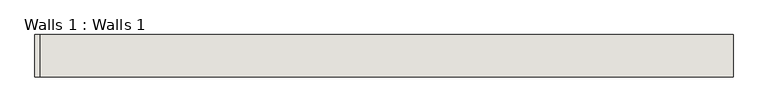
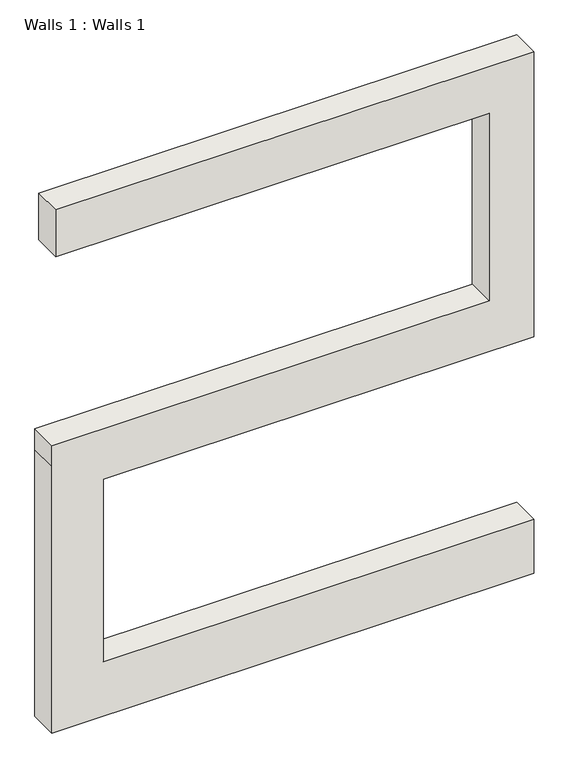
"""IFC4 building model written with IfcOpenShell, lengths in millimetres: wall geometry, Walls 1 : Walls 1."""

from ifc_helpers import new_model, si_unit, frame, origin, place, context, project, spatial, polyline, outline, extrude, source, transform, mapped, element, save


def walls_1_walls_1_82da7aad(model_context):
    return source(origin(), model_context, "Body", "SweptSolid", [
        extrude(outline(polyline([(3124.2671875, -5065.4871298), (3124.2671875, 2101.2415497), (3979.0749524, 2101.2415497), (3979.0749524, -4299.5584503), (6844.0122564, -4299.5584503), (6844.0122564, 2101.2415497), (11327.1268001, 2101.2415497), (11327.1268001, -5008.3371298), (10594.143582, -5008.3371298), (10594.143582, 1437.3335019), (7643.6690266, 1437.3335019), (7643.6690266, -5065.4871298), (7315.2, -5065.4871298), (3124.2671875, -5065.4871298)])), frame((0.0, -50.8786787, 0.0), z_axis=(0.0, 1.0, 0.0), x_axis=(0.0, 0.0, 1.0)), (0.0, 0.0, 1.0), 433.4146605),
    ])


if __name__ == "__main__":
    model = new_model("IFC4")
    model_context = context("Model", 3, world=origin())
    ifc_project = project(units=[si_unit("LENGTHUNIT", "METRE", prefix="MILLI")], contexts=[model_context])
    site = spatial("IfcSite", under=ifc_project)
    building = spatial("IfcBuilding", under=site)
    placement = place(None, origin())
    walls_1_walls_1_shape = walls_1_walls_1_82da7aad(model_context)
    element("IfcWall", 1, ObjectType="Walls 1 : Walls 1", at=placement, inside=building, context=model_context, shape_type="MappedRepresentation", body=[
        mapped(walls_1_walls_1_shape, transform((0.0, 0.0, 0.0), x_axis=(1.0, 0.0, 0.0), y_axis=(0.0, 1.0, 0.0), z_axis=(0.0, 0.0, 1.0))),
    ])
    save(model, "model.ifc")

# Revit data of these elements
# Element 1 (IfcWall, "Walls 1 : Walls 1")
#   Materials on its faces: "Default Wall"
# Materials
#   "Default Wall": colour RGB 128 128 128, transparency 0
